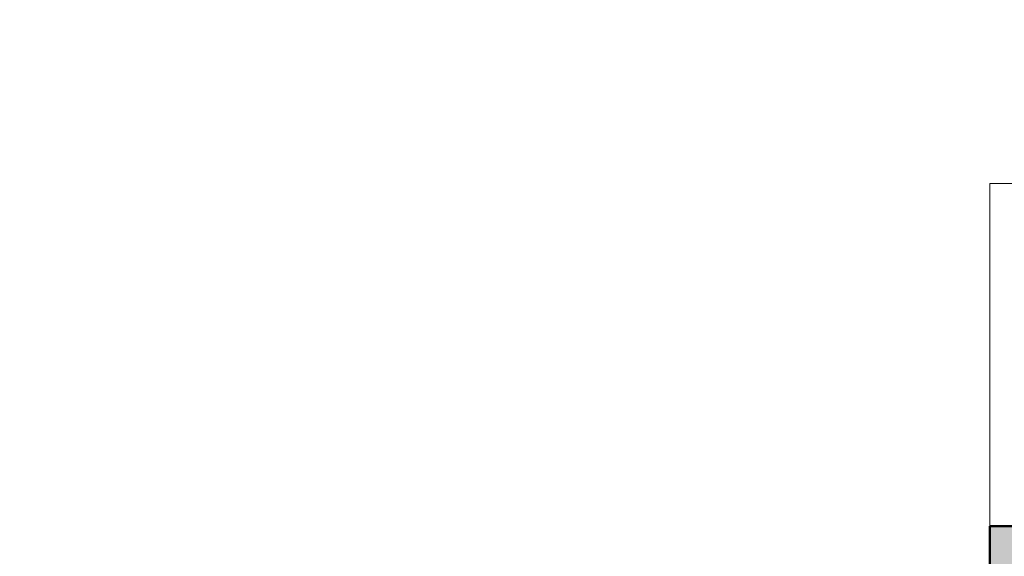
# Model space of a CAD drawing. Units: inches. Extents: x 2307 to 2544, y 2171 to 2540.
# Tile 18 of 52: x 2384 to 2453, y 2317 to 2355. Entities that reach past the tile are written whole.
import ezdxf

# ---------------------------------------------------------------- set-up
doc = ezdxf.new("R2010")
doc.units = ezdxf.units.IN
doc.layers.add('A-FLOR-CASE', color=9, linetype='Continuous', lineweight=18)
doc.layers.add('A-WALL', color=7, linetype='Continuous', lineweight=50)
doc.layers.add('A-WALL-PATT', color=18, linetype='Continuous', lineweight=13, true_color=0x000000)

msp = doc.modelspace()

# ---------------------------------------------------------------- hatches: boundary and pattern name
at = {"layer": 'A-WALL-PATT'}
h = msp.add_hatch(color=256, dxfattribs=at)
h.dxf.hatch_style = 1
h.paths.add_polyline_path([(2433.6935, 2199.5096), (2415.6423, 2199.5096), (2415.6423, 2190.5096), (2433.7832, 2190.5096)], flags=17)
h.paths.add_polyline_path([(2367.6423, 2199.5096), (2335.6958, 2199.5096), (2335.6958, 2307.3983), (2326.6958, 2307.3983), (2326.6958, 2190.5096), (2367.6423, 2190.5096)])
h.paths.add_polyline_path([(2524.6958, 2520.5096), (2496.7832, 2520.5096), (2496.7832, 2515.5149), (2472.7832, 2515.5149), (2472.7832, 2520.5096), (2415.4028, 2520.5096), (2415.4028, 2511.5096), (2451.6958, 2511.5096), (2451.6958, 2439.5096), (2451.6958, 2391.5096), (2445.6958, 2391.5096), (2445.6958, 2387.5096), (2455.6958, 2387.5096), (2455.6958, 2435.5096), (2461.6958, 2435.5096), (2461.6958, 2439.5096), (2455.6958, 2439.5096), (2455.6958, 2511.5096), (2515.6958, 2511.5096), (2515.6958, 2439.5096), (2491.6958, 2439.5096), (2491.6958, 2435.5096), (2515.6958, 2435.5096), (2515.6958, 2319.5096), (2451.6958, 2319.5096), (2451.6958, 2281.5096), (2481.6958, 2281.5096), (2481.6958, 2225.5096), (2485.6958, 2225.5096), (2485.6958, 2285.5096), (2455.6958, 2285.5096), (2455.6958, 2315.5096), (2515.6958, 2315.5096), (2515.6958, 2199.5096), (2469.6952, 2199.5096), (2469.785, 2190.5096), (2524.6958, 2190.5096)])

# ---------------------------------------------------------------- linework, layer by layer
at = {"layer": 'A-FLOR-CASE'}
for p, q in [((2491.6958, 2343.5096), (2451.6958, 2343.5096)), ((2451.6958, 2343.5096), (2451.6958, 2319.5096))]:
    msp.add_line(p, q, dxfattribs=at)
at = {"layer": 'A-WALL'}
for p, q in [((2515.6958, 2319.5096), (2451.6958, 2319.5096)), ((2451.6958, 2319.5096), (2451.6958, 2281.5096))]:
    msp.add_line(p, q, dxfattribs=at)

doc.saveas('drawing.dxf')
